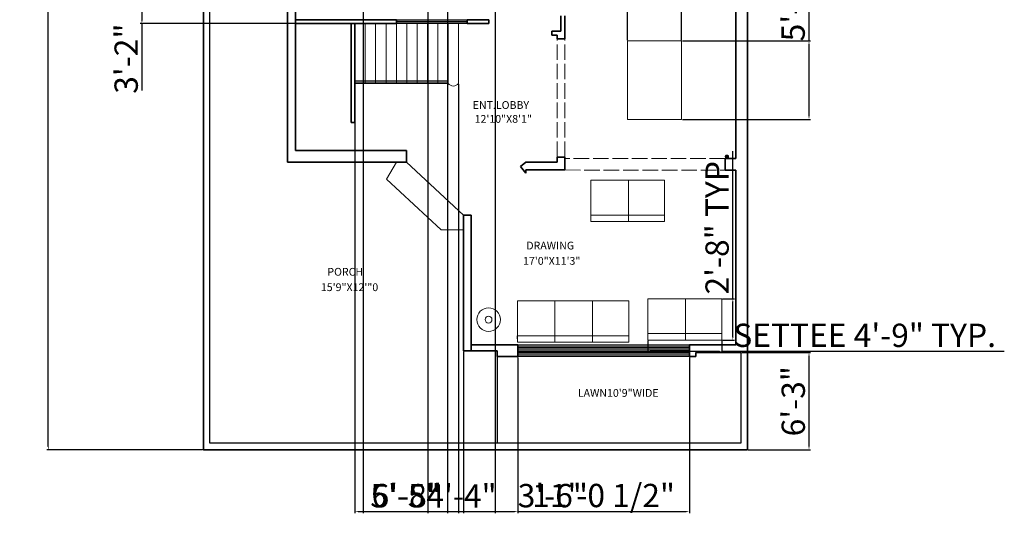
# Model space of a CAD drawing. Units: inches. Extents: x 2484 to 3244, y 1684 to 2692.
# Tile 1 of 3: x 2484 to 3244, y 1684 to 2081. Entities that reach past the tile are written whole.
import ezdxf

# ---------------------------------------------------------------- set-up
doc = ezdxf.new("R2010")
doc.units = ezdxf.units.IN
doc.linetypes.add('ACAD_ISO02W100', pattern=[15, 12, -3])
doc.layers.get('0').update_dxf_attribs({"color": 120})
for name, color, linetype, lineweight in [('A-ANNO-DIMS', 2, 'Continuous', 18), ('A-AREA-IDEN', 2, 'Continuous', 18), ('A-FLOR-STRS', 4, 'Continuous', 18), ('A-FURN', 40, 'Continuous', 18), ('A-GLAZ', 4, 'Continuous', 13), ('A-WALL', 120, 'Continuous', 35), ('A-WALL-OVHD', 255, 'ACAD_ISO02W100', 18), ('C-PROP', 120, 'Continuous', 35), ('C-SITE', 120, 'Continuous', 25)]:
    doc.layers.add(name, color=color, linetype=linetype, lineweight=lineweight)
doc.styles.get("Standard").update_dxf_attribs({"font": 'arial.ttf'})
doc.dimstyles.new('ISO-25', dxfattribs={"dimtxt": 18, "dimasz": 2.5, "dimexe": 1.25, "dimexo": 0.625, "dimtad": 1, "dimdec": 0, "dimlunit": 3, "dimtxsty": 'Standard', "dimcen": 2.5, "dimadec": 0, "dimazin": 0, "dimtfac": 1, "dimtdec": 0, "dimtmove": 0, "dimatfit": 3, "dimfxl": 1, "dimarcsym": 0})

# ---------------------------------------------------------------- blocks, each defined once
blk = doc.blocks.new('*D2')
at = {"layer": 'A-ANNO-DIMS', "color": 0, "lineweight": -2, "transparency": 16777216}
for p, q in [((2625.46, 2528.71), (2505.02, 2528.71)), ((2506.27, 1751.21), (2506.27, 2526.21)), ((2625.46, 1748.71), (2505.02, 1748.71))]:
    blk.add_line(p, q, dxfattribs=at)
at = {"layer": 'A-ANNO-DIMS', "color": 0, "transparency": 16777216}
for points in [[(2505.85, 2526.21), (2506.68, 2526.21), (2506.27, 2528.71)], [(2505.85, 1751.21), (2506.68, 1751.21), (2506.27, 1748.71)]]:
    blk.add_solid(points, dxfattribs=at)
at = {"layer": 'Defpoints', "color": 0, "transparency": 16777216}
for p in [(2506.27, 2528.71), (2626.09, 2528.71), (2626.09, 1748.71)]:
    blk.add_point(p, dxfattribs=at)
at = {"layer": 'A-ANNO-DIMS', "color": 0, "transparency": 16777216, "insert": (2496.45, 2138.71), "char_height": 18, "attachment_point": 5, "rotation": 90}
blk.add_mtext("65'", dxfattribs=at)
blk = doc.blocks.new('SOFA-3')
for p, q in [((0.07, 0), (0.07, 32)), ((0.07, 32), (86.07, 32)), ((29.07, 0), (29.07, 32)), ((58.07, 0), (58.07, 32)), ((86.07, 32), (86.07, 0)), ((0.07, 0), (0, 5)), ((0, 5), (86.07, 5)), ((0.07, 0), (0.07, 5)), ((86.07, 0), (0.07, 0))]:
    blk.add_line(p, q)
blk = doc.blocks.new('SOFA-2')
for p, q in [((0, 0), (0, 32)), ((0, 32), (57, 32)), ((29, 0), (29, 32)), ((57, 32), (57, 0)), ((0, 5), (57, 5)), ((57, 0), (0, 0))]:
    blk.add_line(p, q)
blk = doc.blocks.new('TABLE-ROUND')
for radius in [9.1, 2.6]:
    blk.add_circle((0, 0), radius)
blk = doc.blocks.new('*D9')
at = {"layer": 'A-ANNO-DIMS', "color": 0, "lineweight": -2, "transparency": 16777216}
for p, q in [((2714.44, 2109.91), (2714.44, 2113.27)), ((2716.94, 2112.02), (2730.14, 2112.02)), ((2732.64, 2109.91), (2732.64, 2113.27)), ((2732.64, 2112.02), (3096.69, 2112.02))]:
    blk.add_line(p, q, dxfattribs=at)
at = {"layer": 'A-ANNO-DIMS', "color": 0, "transparency": 16777216}
for points in [[(2716.94, 2112.44), (2716.94, 2111.6), (2714.44, 2112.02)], [(2730.14, 2112.44), (2730.14, 2111.6), (2732.64, 2112.02)]]:
    blk.add_solid(points, dxfattribs=at)
at = {"layer": 'Defpoints', "color": 0, "transparency": 16777216}
for p in [(2714.44, 2109.29), (2732.64, 2112.02), (2732.64, 2109.29)]:
    blk.add_point(p, dxfattribs=at)
at = {"layer": 'A-ANNO-DIMS', "color": 0, "transparency": 16777216, "insert": (2915.92, 2121.96), "char_height": 18, "attachment_point": 5}
blk.add_mtext('ROUND SIDE TABLE 1\'-6" TYP.', dxfattribs=at)
blk = doc.blocks.new('*D15')
at = {"layer": 'A-ANNO-DIMS', "color": 0, "lineweight": -2, "transparency": 16777216}
for p, q in [((2969.26, 1832.75), (2969.26, 1823.57)), ((3026.26, 1832.75), (3026.26, 1823.57)), ((2971.76, 1824.82), (3023.76, 1824.82)), ((3026.26, 1824.82), (3244.44, 1824.82))]:
    blk.add_line(p, q, dxfattribs=at)
at = {"layer": 'A-ANNO-DIMS', "color": 0, "transparency": 16777216}
for points in [[(2971.76, 1825.24), (2971.76, 1824.4), (2969.26, 1824.82)], [(3023.76, 1825.24), (3023.76, 1824.4), (3026.26, 1824.82)]]:
    blk.add_solid(points, dxfattribs=at)
at = {"layer": 'Defpoints', "color": 0, "transparency": 16777216}
for p in [(2969.26, 1833.37), (3026.26, 1833.37), (3026.26, 1824.82)]:
    blk.add_point(p, dxfattribs=at)
at = {"layer": 'A-ANNO-DIMS', "color": 0, "transparency": 16777216, "insert": (3136.6, 1834.75), "char_height": 18, "attachment_point": 5}
blk.add_mtext('SETTEE 4\'-9" TYP.', dxfattribs=at)
blk = doc.blocks.new('*D16')
at = {"layer": 'A-ANNO-DIMS', "color": 0, "lineweight": -2, "transparency": 16777216}
for p, q in [((3034.81, 1865.37), (3034.81, 1979.15)), ((3026.89, 1865.37), (3036.06, 1865.37)), ((3034.81, 1835.87), (3034.81, 1862.87)), ((3026.89, 1833.37), (3036.06, 1833.37))]:
    blk.add_line(p, q, dxfattribs=at)
at = {"layer": 'A-ANNO-DIMS', "color": 0, "transparency": 16777216}
for points in [[(3034.4, 1862.87), (3035.23, 1862.87), (3034.81, 1865.37)], [(3034.4, 1835.87), (3035.23, 1835.87), (3034.81, 1833.37)]]:
    blk.add_solid(points, dxfattribs=at)
at = {"layer": 'Defpoints', "color": 0, "transparency": 16777216}
for p in [(3026.26, 1865.37), (3034.81, 1865.37), (3026.26, 1833.37)]:
    blk.add_point(p, dxfattribs=at)
at = {"layer": 'A-ANNO-DIMS', "color": 0, "transparency": 16777216, "insert": (3025, 1923.51), "char_height": 18, "attachment_point": 5, "rotation": 90}
blk.add_mtext('2\'-8" TYP.', dxfattribs=at)
blk = doc.blocks.new('*D21')
at = {"layer": 'A-ANNO-DIMS', "color": 0, "lineweight": -2, "transparency": 16777216}
for p, q in [((2749.51, 2385.09), (2749.51, 1699.91)), ((2814.51, 2385.09), (2814.51, 1699.91)), ((2752.01, 1701.16), (2812.01, 1701.16))]:
    blk.add_line(p, q, dxfattribs=at)
at = {"layer": 'A-ANNO-DIMS', "color": 0, "transparency": 16777216}
for points in [[(2752.01, 1701.58), (2752.01, 1700.75), (2749.51, 1701.16)], [(2812.01, 1701.58), (2812.01, 1700.75), (2814.51, 1701.16)]]:
    blk.add_solid(points, dxfattribs=at)
at = {"layer": 'Defpoints', "color": 0, "transparency": 16777216}
for p in [(2749.51, 2385.71), (2814.51, 2385.71), (2814.51, 1701.16)]:
    blk.add_point(p, dxfattribs=at)
at = {"layer": 'A-ANNO-DIMS', "color": 0, "transparency": 16777216, "insert": (2782.01, 1710.94), "char_height": 18, "attachment_point": 5}
blk.add_mtext('5\'-5"', dxfattribs=at)
blk = doc.blocks.new('*D23')
at = {"layer": 'A-ANNO-DIMS', "color": 0, "lineweight": -2, "transparency": 16777216}
for p, q in [((2953.42, 2064.92), (2953.42, 2577.51)), ((2995.24, 2064.92), (2995.24, 2577.51)), ((2955.92, 2576.26), (2992.74, 2576.26)), ((2995.24, 2576.26), (3046.83, 2576.26))]:
    blk.add_line(p, q, dxfattribs=at)
at = {"layer": 'A-ANNO-DIMS', "color": 0, "transparency": 16777216}
for points in [[(2955.92, 2576.68), (2955.92, 2575.85), (2953.42, 2576.26)], [(2992.74, 2576.68), (2992.74, 2575.85), (2995.24, 2576.26)]]:
    blk.add_solid(points, dxfattribs=at)
at = {"layer": 'Defpoints', "color": 0, "transparency": 16777216}
for p in [(2995.24, 2576.26), (2953.42, 2064.3), (2995.24, 2064.3)]:
    blk.add_point(p, dxfattribs=at)
at = {"layer": 'A-ANNO-DIMS', "color": 0, "transparency": 16777216, "insert": (3022.28, 2586.08), "char_height": 18, "attachment_point": 5}
blk.add_mtext('3\'-6"', dxfattribs=at)
blk = doc.blocks.new('*D24')
at = {"layer": 'A-ANNO-DIMS', "color": 0, "lineweight": -2, "transparency": 16777216}
for p, q in [((3093.64, 2064.3), (3093.64, 2157.84)), ((2995.86, 2064.3), (3094.89, 2064.3)), ((3093.64, 2006.27), (3093.64, 2061.8)), ((2995.86, 2003.77), (3094.89, 2003.77))]:
    blk.add_line(p, q, dxfattribs=at)
at = {"layer": 'A-ANNO-DIMS', "color": 0, "transparency": 16777216}
for points in [[(3093.22, 2061.8), (3094.05, 2061.8), (3093.64, 2064.3)], [(3093.22, 2006.27), (3094.05, 2006.27), (3093.64, 2003.77)]]:
    blk.add_solid(points, dxfattribs=at)
at = {"layer": 'Defpoints', "color": 0, "transparency": 16777216}
for p in [(2995.24, 2064.3), (3093.64, 2064.3), (2995.24, 2003.77)]:
    blk.add_point(p, dxfattribs=at)
at = {"layer": 'A-ANNO-DIMS', "color": 0, "transparency": 16777216, "insert": (3083.71, 2112.32), "char_height": 18, "attachment_point": 5, "rotation": 90}
blk.add_mtext('5\'-0 1/2"', dxfattribs=at)
blk = doc.blocks.new('*D28')
at = {"layer": 'A-ANNO-DIMS', "color": 0, "lineweight": -2, "transparency": 16777216}
for p, q in [((2690.46, 2115.7), (2577.29, 2115.7)), ((2578.54, 2113.2), (2578.54, 2080.21)), ((2696.46, 2077.71), (2577.29, 2077.71)), ((2578.54, 2077.71), (2578.54, 2026.13))]:
    blk.add_line(p, q, dxfattribs=at)
at = {"layer": 'A-ANNO-DIMS', "color": 0, "transparency": 16777216}
for points in [[(2578.12, 2113.2), (2578.95, 2113.2), (2578.54, 2115.7)], [(2578.12, 2080.21), (2578.95, 2080.21), (2578.54, 2077.71)]]:
    blk.add_solid(points, dxfattribs=at)
at = {"layer": 'Defpoints', "color": 0, "transparency": 16777216}
for p in [(2691.09, 2115.7), (2578.54, 2077.71), (2697.09, 2077.71)]:
    blk.add_point(p, dxfattribs=at)
at = {"layer": 'A-ANNO-DIMS', "color": 0, "transparency": 16777216, "insert": (2568.72, 2050.67), "char_height": 18, "attachment_point": 5, "rotation": 90}
blk.add_mtext('3\'-2"', dxfattribs=at)
blk = doc.blocks.new('*D29')
at = {"layer": 'A-ANNO-DIMS', "color": 0, "lineweight": -2, "transparency": 16777216}
for p, q in [((2868.8, 1820.09), (2868.8, 1699.91)), ((3001.3, 1820.09), (3001.3, 1699.91)), ((2871.3, 1701.16), (2998.8, 1701.16))]:
    blk.add_line(p, q, dxfattribs=at)
at = {"layer": 'A-ANNO-DIMS', "color": 0, "transparency": 16777216}
for points in [[(2871.3, 1701.58), (2871.3, 1700.75), (2868.8, 1701.16)], [(2998.8, 1701.58), (2998.8, 1700.75), (3001.3, 1701.16)]]:
    blk.add_solid(points, dxfattribs=at)
at = {"layer": 'Defpoints', "color": 0, "transparency": 16777216}
for p in [(2868.8, 1820.71), (3001.3, 1820.71), (3001.3, 1701.16)]:
    blk.add_point(p, dxfattribs=at)
at = {"layer": 'A-ANNO-DIMS', "color": 0, "transparency": 16777216, "insert": (2935.05, 1711.1), "char_height": 18, "attachment_point": 5}
blk.add_mtext('11\'-0 1/2"', dxfattribs=at)
blk = doc.blocks.new('*D30')
at = {"layer": 'A-ANNO-DIMS', "color": 0, "lineweight": -2, "transparency": 16777216}
for p, q in [((2826.8, 1824.59), (2826.8, 1699.91)), ((2868.8, 1820.09), (2868.8, 1699.91)), ((2829.3, 1701.16), (2866.3, 1701.16)), ((2868.8, 1701.16), (2920.39, 1701.16))]:
    blk.add_line(p, q, dxfattribs=at)
at = {"layer": 'A-ANNO-DIMS', "color": 0, "transparency": 16777216}
for points in [[(2829.3, 1701.58), (2829.3, 1700.75), (2826.8, 1701.16)], [(2866.3, 1701.58), (2866.3, 1700.75), (2868.8, 1701.16)]]:
    blk.add_solid(points, dxfattribs=at)
at = {"layer": 'Defpoints', "color": 0, "transparency": 16777216}
for p in [(2826.8, 1825.21), (2868.8, 1820.71), (2868.8, 1701.16)]:
    blk.add_point(p, dxfattribs=at)
at = {"layer": 'A-ANNO-DIMS', "color": 0, "transparency": 16777216, "insert": (2895.84, 1710.98), "char_height": 18, "attachment_point": 5}
blk.add_mtext('3\'-6"', dxfattribs=at)
blk = doc.blocks.new('*D36')
at = {"layer": 'A-ANNO-DIMS', "color": 0, "lineweight": -2, "transparency": 16777216}
for p, q in [((3041.71, 1823.71), (3094.89, 1823.71)), ((3093.64, 1751.21), (3093.64, 1821.21)), ((3046.71, 1748.71), (3094.89, 1748.71))]:
    blk.add_line(p, q, dxfattribs=at)
at = {"layer": 'A-ANNO-DIMS', "color": 0, "transparency": 16777216}
for points in [[(3093.22, 1821.21), (3094.05, 1821.21), (3093.64, 1823.71)], [(3093.22, 1751.21), (3094.05, 1751.21), (3093.64, 1748.71)]]:
    blk.add_solid(points, dxfattribs=at)
at = {"layer": 'Defpoints', "color": 0, "transparency": 16777216}
for p in [(3041.09, 1823.71), (3093.64, 1823.71), (3046.09, 1748.71)]:
    blk.add_point(p, dxfattribs=at)
at = {"layer": 'A-ANNO-DIMS', "color": 0, "transparency": 16777216, "insert": (3083.82, 1786.21), "char_height": 18, "attachment_point": 5, "rotation": 90}
blk.add_mtext('6\'-3"', dxfattribs=at)
blk = doc.blocks.new('*D37')
at = {"layer": 'A-ANNO-DIMS', "color": 0, "lineweight": -2, "transparency": 16777216}
for p, q in [((2799.42, 2313.09), (2799.42, 1699.91)), ((2851.28, 2313.09), (2851.28, 1699.91)), ((2801.92, 1701.16), (2848.78, 1701.16))]:
    blk.add_line(p, q, dxfattribs=at)
at = {"layer": 'A-ANNO-DIMS', "color": 0, "transparency": 16777216}
for points in [[(2801.92, 1701.58), (2801.92, 1700.75), (2799.42, 1701.16)], [(2848.78, 1701.58), (2848.78, 1700.75), (2851.28, 1701.16)]]:
    blk.add_solid(points, dxfattribs=at)
at = {"layer": 'Defpoints', "color": 0, "transparency": 16777216}
for p in [(2799.42, 2313.71), (2851.28, 2313.71), (2851.28, 1701.16)]:
    blk.add_point(p, dxfattribs=at)
at = {"layer": 'A-ANNO-DIMS', "color": 0, "transparency": 16777216, "insert": (2825.35, 1710.79), "char_height": 18, "attachment_point": 5}
blk.add_mtext('4\'-4"', dxfattribs=at)
blk = doc.blocks.new('*D38')
at = {"layer": 'A-ANNO-DIMS', "color": 0, "lineweight": -2, "transparency": 16777216}
for p, q in [((2743.04, 2030.91), (2743.04, 1699.91)), ((2823.04, 2030.91), (2823.04, 1699.91)), ((2745.54, 1701.16), (2820.54, 1701.16))]:
    blk.add_line(p, q, dxfattribs=at)
at = {"layer": 'A-ANNO-DIMS', "color": 0, "transparency": 16777216}
for points in [[(2745.54, 1701.58), (2745.54, 1700.75), (2743.04, 1701.16)], [(2820.54, 1701.58), (2820.54, 1700.75), (2823.04, 1701.16)]]:
    blk.add_solid(points, dxfattribs=at)
at = {"layer": 'Defpoints', "color": 0, "transparency": 16777216}
for p in [(2743.04, 2031.54), (2823.04, 2031.54), (2823.04, 1701.16)]:
    blk.add_point(p, dxfattribs=at)
at = {"layer": 'A-ANNO-DIMS', "color": 0, "transparency": 16777216, "insert": (2783.04, 1710.98), "char_height": 18, "attachment_point": 5}
blk.add_mtext('6\'-8"', dxfattribs=at)

msp = doc.modelspace()

# ---------------------------------------------------------------- linework, layer by layer
at = {"layer": 'A-FLOR-STRS'}
for p, q in [((2743.04, 2077.71), (2751.04, 2077.71)), ((2751.04, 2077.71), (2751.04, 2031.54)), ((2759.04, 2077.71), (2759.04, 2031.54)), ((2767.04, 2077.71), (2767.04, 2031.54)), ((2775.04, 2077.71), (2775.04, 2031.54)), ((2783.04, 2077.71), (2783.04, 2031.54)), ((2791.04, 2077.71), (2791.04, 2031.54)), ((2799.04, 2077.71), (2799.04, 2031.54)), ((2807.04, 2077.71), (2807.04, 2031.54)), ((2815.04, 2077.71), (2815.04, 2031.54)), ((2823.04, 2077.71), (2823.04, 2031.54)), ((2743.04, 2033.54), (2815.04, 2033.54)), ((2743.04, 2032.54), (2815.04, 2032.54)), ((2743.04, 2031.54), (2815.04, 2031.54)), ((2775.23, 1970.71), (2767.53, 1957.5)), ((2826.8, 1929.9), (2782.98, 1970.71)), ((2767.53, 1957.5), (2809.68, 1918.62)), ((2809.68, 1918.62), (2826.8, 1918.62))]:
    msp.add_line(p, q, dxfattribs=at)
msp.add_arc((2819.04, 2034.54), 5, 216.8699, 323.1301, dxfattribs=at)
at = {"layer": 'A-FURN'}
msp.add_lwpolyline([(2953.42, 2064.3), (2995.24, 2064.3), (2995.24, 2003.77), (2953.42, 2003.77)], close=True, dxfattribs=at)
at = {"layer": 'A-GLAZ'}
for p, q in [((2775.25, 2080.71), (2829.81, 2080.71)), ((2775.25, 2079.71), (2829.81, 2079.71)), ((2775.25, 2078.71), (2829.81, 2078.71)), ((2775.25, 2077.71), (2829.81, 2077.71)), ((2868.8, 1829.71), (3001.3, 1829.71)), ((2868.8, 1828.71), (3001.3, 1828.71)), ((2868.8, 1827.71), (3001.3, 1827.71)), ((2868.8, 1826.71), (3001.3, 1826.71)), ((2868.8, 1825.71), (3001.3, 1825.71)), ((2868.8, 1824.71), (3001.3, 1824.71)), ((2868.8, 1823.71), (3001.3, 1823.71)), ((2868.8, 1822.71), (3001.3, 1822.71)), ((2868.8, 1821.71), (3001.3, 1821.71)), ((2868.8, 1820.71), (3001.3, 1820.71))]:
    msp.add_line(p, q, dxfattribs=at)
at = {"layer": 'A-WALL'}
for p, q in [((3037.09, 2397.94), (3037.09, 1973.56)), ((2691.09, 1970.71), (2691.09, 2115.7)), ((2697.09, 1979.71), (2697.09, 2115.7)), ((2902.09, 2083.7), (2902.09, 2071.85)), ((2905.09, 2083.7), (2905.09, 2065.85)), ((2775.25, 2080.71), (2697.09, 2080.71)), ((2775.25, 2077.71), (2697.09, 2077.71)), ((2740.04, 2077.71), (2740.04, 2001.4)), ((2743.04, 2001.4), (2743.04, 2077.71)), ((2775.25, 2080.71), (2775.25, 2077.71)), ((2829.81, 2080.71), (2846.5, 2080.71)), ((2829.81, 2080.71), (2829.81, 2077.71)), ((2846.5, 2077.71), (2829.81, 2077.71)), ((2846.5, 2080.71), (2846.5, 2077.71)), ((2895.09, 2068.85), (2895.09, 2071.85)), ((2895.09, 2071.85), (2902.09, 2071.85)), ((2899.09, 2068.85), (2895.09, 2068.85)), ((2899.09, 2065.85), (2899.09, 2068.85)), ((2902.09, 2065.85), (2899.09, 2065.85)), ((2905.09, 2065.85), (2902.09, 2065.85)), ((2740.04, 2001.4), (2743.04, 2001.4)), ((2782.98, 1979.71), (2697.09, 1979.71)), ((2782.98, 1970.71), (2782.98, 1979.71)), ((2697.09, 1970.71), (2691.09, 1970.71)), ((2782.98, 1970.71), (2697.09, 1970.71)), ((2875.09, 1970.71), (2870.91, 1967.44)), ((2899.09, 1970.71), (2875.09, 1970.71)), ((2902.09, 1974.71), (2899.09, 1974.71)), ((2899.09, 1974.71), (2899.09, 1970.71)), ((2902.09, 1974.71), (2905.09, 1974.71)), ((2905.09, 1974.71), (2905.09, 1964.71)), ((3028.9, 1973.56), (3028.89, 1964.57)), ((3037.09, 1973.56), (3028.9, 1973.56)), ((2870.91, 1967.44), (2874.91, 1962.32)), ((2874.91, 1962.32), (2874.91, 1964.71)), ((2874.91, 1964.71), (2902.09, 1964.71)), ((2902.09, 1964.71), (2905.09, 1964.71)), ((3028.89, 1964.57), (3037.09, 1964.56)), ((3037.09, 1964.56), (3037.09, 1832.71)), ((2832.8, 1929.9), (2826.8, 1929.9)), ((2826.8, 1929.9), (2826.8, 1825.21)), ((2832.8, 1929.9), (2832.8, 1825.21)), ((3037.09, 1829.71), (3037.09, 1832.71)), ((2852.8, 1825.21), (2826.8, 1825.21)), ((2868.8, 1829.71), (2832.8, 1829.71)), ((2832.8, 1829.71), (2868.8, 1829.71)), ((2852.8, 1820.71), (2852.8, 1825.21)), ((2868.8, 1829.71), (2868.8, 1820.71)), ((3001.3, 1820.71), (3001.3, 1829.71)), ((3001.3, 1829.71), (3037.09, 1829.71)), ((2868.8, 1820.71), (2852.8, 1820.71)), ((3001.3, 1820.71), (3006.3, 1820.71)), ((3006.3, 1823.71), (3037.09, 1823.71)), ((3006.3, 1820.71), (3006.3, 1823.71)), ((3037.09, 1823.71), (3041.09, 1823.71))]:
    msp.add_line(p, q, dxfattribs=at)
at = {"layer": 'A-WALL-OVHD'}
for p, q in [((2899.09, 1974.71), (2899.09, 2065.85)), ((2905.09, 1974.71), (2905.09, 2065.85)), ((3028.9, 1973.56), (2905.09, 1973.56)), ((2905.09, 1964.71), (3028.89, 1964.57))]:
    msp.add_line(p, q, dxfattribs=at)
at = {"layer": 'C-PROP'}
msp.add_lwpolyline([(2626.09, 2528.71), (3046.09, 2528.71), (3046.09, 1748.71), (2626.09, 1748.71)], close=True, dxfattribs=at)
at = {"layer": 'C-SITE'}
for p, q in [((2631.09, 1753.71), (2631.09, 2523.71)), ((2852.8, 1820.71), (2852.8, 1753.71)), ((3041.09, 1823.71), (3041.09, 1753.71)), ((3041.09, 1753.71), (2631.09, 1753.71))]:
    msp.add_line(p, q, dxfattribs=at)

# ---------------------------------------------------------------- block references
at = {"layer": 'A-FURN'}
for name, p in [('SOFA-2', (2925.14, 1924.93)), ('SOFA-3', (2868.39, 1831.79)), ('SOFA-2', (2969.26, 1833.37)), ('TABLE-ROUND', (2846.24, 1849.19))]:
    msp.add_blockref(name, p, dxfattribs=at)

# ---------------------------------------------------------------- texts
at = {"layer": 'A-AREA-IDEN'}
for tag, p in [('ENT.LOBBY', (2833.97, 2011.86)), ('12\'10"X8\'1"', (2835.45, 2001.14)), ('DRAWING', (2875.36, 1903.36)), ('17\'0"X11\'3"', (2872.87, 1891.54)), ('PORCH', (2721.76, 1883.11)), ('15\'9"X12\'"0', (2716.75, 1871.23)), ('LAWN10\'9"WIDE', (2915.16, 1789.61))]:
    msp.add_attdef(tag, p, '', height=6, dxfattribs=at)

# ---------------------------------------------------------------- dimensions: what is measured, and where the dimension line sits
at = {"layer": 'A-ANNO-DIMS'}
for base, p1, p2, picture, middle in [((2995.24, 2576.26), (2953.42, 2064.3), (2995.24, 2064.3), '*D23', (3022.28, 2586.08)), ((2814.51, 1701.16), (2749.51, 2385.71), (2814.51, 2385.71), '*D21', (2782.01, 1710.94)), ((2851.28, 1701.16), (2799.42, 2313.71), (2851.28, 2313.71), '*D37', (2825.35, 1710.79)), ((2823.04, 1701.16), (2743.04, 2031.54), (2823.04, 2031.54), '*D38', (2783.04, 1710.98)), ((2868.8, 1701.16), (2826.8, 1825.21), (2868.8, 1820.71), '*D30', (2895.84, 1710.98)), ((3001.3, 1701.16), (2868.8, 1820.71), (3001.3, 1820.71), '*D29', (2935.05, 1711.1))]:
    dim = msp.add_linear_dim(base=base, p1=p1, p2=p2, dimstyle='ISO-25', override={"dimdec": 1, "dimlfac": 1, "dimrnd": 0, "dimzin": 1, "dimdsep": 46, "dimlunit": 4, "dimfrac": 2}, dxfattribs=at)
    dim.commit()
    dim.dimension.update_dxf_attribs({"geometry": picture, "text_midpoint": middle})
for base, p1, p2, override, picture, middle in [((2506.27, 2528.71), (2626.09, 1748.71), (2626.09, 2528.71), {"dimclrd": 0, "dimclre": 0, "dimclrt": 0}, '*D2', (2496.45, 2138.71)), ((3093.64, 2064.3), (2995.24, 2003.77), (2995.24, 2064.3), {"dimdec": 1, "dimlfac": 1, "dimrnd": 0, "dimzin": 1, "dimdsep": 46, "dimlunit": 4, "dimfrac": 2}, '*D24', (3083.71, 2112.32)), ((2578.54, 2077.71), (2691.09, 2115.7), (2697.09, 2077.71), {"dimdec": 1, "dimlfac": 1, "dimrnd": 0, "dimzin": 1, "dimdsep": 46, "dimlunit": 4, "dimfrac": 2}, '*D28', (2568.72, 2050.67)), ((3093.64, 1823.71), (3046.09, 1748.71), (3041.09, 1823.71), {"dimdec": 1, "dimlfac": 1, "dimrnd": 0, "dimzin": 1, "dimdsep": 46, "dimlunit": 4, "dimfrac": 2}, '*D36', (3083.82, 1786.21))]:
    dim = msp.add_linear_dim(base=base, p1=p1, p2=p2, angle=90, dimstyle='ISO-25', override=override, dxfattribs=at)
    dim.commit()
    dim.dimension.update_dxf_attribs({"geometry": picture, "text_midpoint": middle})
for base, p1, p2, text, picture, middle in [((2732.64, 2112.02), (2714.44, 2109.29), (2732.64, 2109.29), 'ROUND SIDE TABLE <> TYP.', '*D9', (2915.92, 2121.96)), ((3026.26, 1824.82), (2969.26, 1833.37), (3026.26, 1833.37), 'SETTEE <> TYP.', '*D15', (3136.6, 1834.75))]:
    dim = msp.add_linear_dim(base=base, p1=p1, p2=p2, text=text, dimstyle='ISO-25', override={"dimdec": 1, "dimlfac": 1, "dimrnd": 0, "dimzin": 1, "dimdsep": 46, "dimlunit": 4, "dimfrac": 2}, dxfattribs=at)
    dim.commit()
    dim.dimension.update_dxf_attribs({"geometry": picture, "text_midpoint": middle})
dim = msp.add_linear_dim(base=(3034.81, 1865.37), p1=(3026.26, 1833.37), p2=(3026.26, 1865.37), angle=90, text='<> TYP.', dimstyle='ISO-25', override={"dimdec": 1, "dimlfac": 1, "dimrnd": 0, "dimzin": 1, "dimdsep": 46, "dimlunit": 4, "dimfrac": 2}, dxfattribs=at)
dim.commit()
dim.dimension.update_dxf_attribs({"geometry": '*D16', "text_midpoint": (3025, 1923.51)})

doc.saveas('drawing.dxf')
